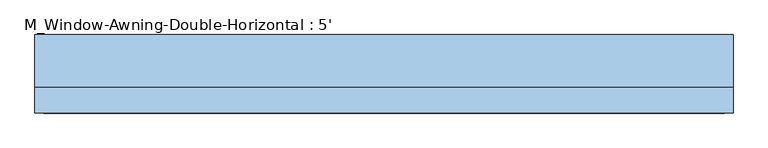
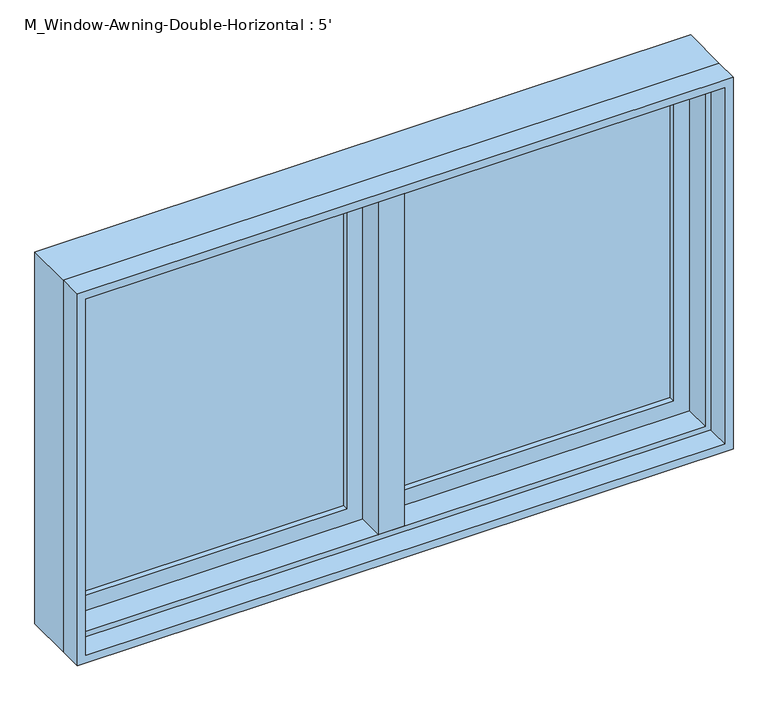
"""IFC4 building model written with IfcOpenShell, lengths in millimetres: window geometry, M_Window-Awning-Double-Horizontal : 5'."""

from ifc_helpers import new_model, si_unit, frame, origin, place, context, project, spatial, polyline, outline, extrude, faceted_brep, source, transform, mapped, element, save


def m_window_awning_double_horizontal_5_337400f2(model_context):
    return source(origin(), model_context, "Body", "SolidModel", [
        faceted_brep([(730.25, 44.45, 1782.65), (730.25, -19.05, 1782.65), (-730.25, -19.05, 1782.65), (-730.25, 44.45, 1782.65), (749.3, 95.25, 1801.7), (749.3, 44.45, 1801.7), (-749.3, 44.45, 1801.7), (-749.3, 95.25, 1801.7), (762.0, -19.05, 1814.4), (762.0, 95.25, 1814.4), (-762.0, 95.25, 1814.4), (-762.0, -19.05, 1814.4), (-730.25, -19.05, 931.75), (-730.25, 44.45, 931.75), (-749.3, 44.45, 912.7), (-749.3, 95.25, 912.7), (-762.0, 95.25, 900.0), (-762.0, -19.05, 900.0), (730.25, -19.05, 931.75), (730.25, 44.45, 931.75), (749.3, 44.45, 912.7), (749.3, 95.25, 912.7), (762.0, 95.25, 900.0), (762.0, -19.05, 900.0)], [[[0, 1, 2, 3]], [[4, 5, 6, 7]], [[8, 9, 10, 11]], [[3, 2, 12, 13]], [[7, 6, 14, 15]], [[11, 10, 16, 17]], [[13, 12, 18, 19]], [[15, 14, 20, 21]], [[17, 16, 22, 23]], [[11, 17, 23, 8], [1, 18, 12, 2]], [[19, 18, 1, 0]], [[5, 20, 14, 6], [3, 13, 19, 0]], [[21, 20, 5, 4]], [[23, 22, 9, 8]], [[9, 22, 16, 10], [7, 15, 21, 4]]]),
        extrude(outline(polyline([(1814.4, -762.0), (900.0, -762.0), (900.0, 762.0), (1814.4, 762.0), (1814.4, -762.0)]), holes=[polyline([(1795.35, 742.95), (919.05, 742.95), (919.05, -742.95), (1795.35, -742.95), (1795.35, 742.95)])]), frame((0.0, -76.2, 0.0), z_axis=(0.0, 1.0, 0.0), x_axis=(0.0, 0.0, 1.0)), (0.0, 0.0, 1.0), 57.15),
        extrude(outline(polyline([(912.7, 749.3), (1801.7, 749.3), (1801.7, 9.525), (912.7, 9.525), (912.7, 749.3)]), holes=[polyline([(969.85, 66.675), (1744.55, 66.675), (1744.55, 692.15), (969.85, 692.15), (969.85, 66.675)])]), frame((0.0, 44.45, 0.0), z_axis=(0.0, 1.0, 0.0), x_axis=(0.0, 0.0, 1.0)), (0.0, 0.0, 1.0), 44.45),
        extrude(outline(polyline([(1801.7, -749.3), (912.7, -749.3), (912.7, -9.525), (1801.7, -9.525), (1801.7, -749.3)]), holes=[polyline([(1744.55, -66.675), (969.85, -66.675), (969.85, -692.15), (1744.55, -692.15), (1744.55, -66.675)])]), frame((0.0, 44.45, 0.0), z_axis=(0.0, 1.0, 0.0), x_axis=(0.0, 0.0, 1.0)), (0.0, 0.0, 1.0), 44.45),
        extrude(outline(polyline([(692.15, 76.2), (692.15, 69.85), (66.675, 69.85), (66.675, 76.2), (692.15, 76.2)])), frame((0.0, 0.0, 969.85), z_axis=(0.0, 0.0, 1.0), x_axis=(1.0, 0.0, 0.0)), (0.0, 0.0, 1.0), 774.7),
        extrude(outline(polyline([(66.675, 57.15), (66.675, 63.5), (692.15, 63.5), (692.15, 57.15), (66.675, 57.15)])), frame((0.0, 0.0, 969.85), z_axis=(0.0, 0.0, 1.0), x_axis=(1.0, 0.0, 0.0)), (0.0, 0.0, 1.0), 774.7),
        extrude(outline(polyline([(-66.675, 76.2), (-66.675, 69.85), (-692.15, 69.85), (-692.15, 76.2), (-66.675, 76.2)])), frame((0.0, 0.0, 969.85), z_axis=(0.0, 0.0, 1.0), x_axis=(1.0, 0.0, 0.0)), (0.0, 0.0, 1.0), 774.7),
        extrude(outline(polyline([(-692.15, 57.15), (-692.15, 63.5), (-66.675, 63.5), (-66.675, 57.15), (-692.15, 57.15)])), frame((0.0, 0.0, 969.85), z_axis=(0.0, 0.0, 1.0), x_axis=(1.0, 0.0, 0.0)), (0.0, 0.0, 1.0), 774.7),
        faceted_brep([(9.525, 95.25, 1801.7), (-9.525, 95.25, 1801.7), (-9.525, 44.45, 1801.7), (9.525, 44.45, 1801.7), (9.525, 95.25, 912.7), (9.525, 44.45, 912.7), (-9.525, 44.45, 912.7), (-9.525, 95.25, 912.7), (-9.525, 44.45, 931.75), (-9.525, 44.45, 1782.65), (-30.1625, 44.45, 931.75), (-30.1625, 44.45, 1782.65), (-30.1625, -19.05, 931.75), (-30.1625, -19.05, 1782.65), (30.1625, -19.05, 931.75), (30.1625, -19.05, 1782.65), (30.1625, 44.45, 931.75), (30.1625, 44.45, 1782.65), (9.525, 44.45, 931.75), (9.525, 44.45, 1782.65)], [[[0, 1, 2, 3]], [[4, 5, 6, 7]], [[1, 0, 4, 7]], [[2, 1, 7, 6, 8, 9]], [[9, 8, 10, 11]], [[11, 10, 12, 13]], [[13, 12, 14, 15]], [[15, 14, 16, 17]], [[17, 16, 18, 19]], [[0, 3, 19, 18, 5, 4]], [[18, 8, 6, 5]], [[9, 19, 3, 2]], [[8, 18, 16, 14, 12, 10]], [[19, 9, 11, 13, 15, 17]]]),
    ])


if __name__ == "__main__":
    model = new_model("IFC4")
    model_context = context("Model", 3, world=origin())
    ifc_project = project(units=[si_unit("LENGTHUNIT", "METRE", prefix="MILLI")], contexts=[model_context])
    site = spatial("IfcSite", under=ifc_project)
    building = spatial("IfcBuilding", under=site)
    placement = place(None, origin())
    m_window_awning_double_horizontal_5_shape = m_window_awning_double_horizontal_5_337400f2(model_context)
    element("IfcWindow", 1, ObjectType="M_Window-Awning-Double-Horizontal : 5'", at=placement, inside=building, context=model_context, shape_type="MappedRepresentation", body=[
        mapped(m_window_awning_double_horizontal_5_shape, transform((0.0, 0.0, 0.0), x_axis=(1.0, 0.0, 0.0), y_axis=(0.0, 1.0, 0.0), z_axis=(0.0, 0.0, 1.0))),
    ])
    save(model, "model.ifc")

# Revit data of these elements
# Type "M_Window-Awning-Double-Horizontal : 5'"
#   Type Mark = "19"
#   Fire Rating = "0.5h"
#   Assembly Code = "B2020100"
#   Analytic Construction = "Double glazing - domestic"
#   Window Inset [instance default] = 0' - 0"
#   Wall Thickness [instance default] = 0' - 5.90551"
#   Interior Wall Closure [instance default] = 0' - 2.15551"
#   Half Width = 2' - 6"
#   Visual Light Transmittance = 0.81
#   Thermal Resistance (R) = 1.8146 (h·ft²·°F)/BTU
#   Solar Heat Gain Coefficient = 0.76
#   Rough Width = 5' - 0.59055"
#   Rough Height = 3' - 0.59055"
#   Height = 3' - 0"
#   Heat Transfer Coefficient (U) = 0.5511 BTU/(h·ft²·°F)
#   Frame Extension [instance default] = 0' - 0 1/4"
#   Exterior Wall Closure [instance default] = 0' - 1 1/4"
#   Extension Jamb [instance default] = 0' - 2.15551"
#   Default Sill Height = 2' - 11.43307"
#   Width = 5' - 0"
#   Muntin Visibility = yes
#   Interior Trim Visibility [instance default] = yes
#   Exterior Trim Visibility [instance default] = yes
#   Extension Jamb Visibility [instance default] = yes
#   Interior Trim Material = Wood - Stained
#   Muntin Pattern = M_Muntin Pattern_2x2 : M_Muntin Pattern_2x2
#   Interior Trim = M_Trim-Window-Interior-Flat : Picture Frame
#   Interior Frame Material = Wood - Stained
#   Glass Panel Material = Glass
#   Exterior Trim Material = Clad - White
#   Exterior Trim = M_Trim-Window-Exterior-Flat : with Sill
#   Exterior Frame Material = Clad - White
#   Wall Closure = (empty or 0)
# Element 1 (IfcWindow, "M_Window-Awning-Double-Horizontal : 5'")
#   Wall Thickness = 0' - 6"
#   Extension Jamb = 0' - 2 1/4"
#   Materials on its faces: "Wood - Stained", "Glass", "Clad - White"
# Materials
#   "Wood - Stained": class "Wood", colour RGB 224 178 126, transparency 0, Cost = 0
#   "Glass": class "Glass", colour RGB 0 128 192, transparency 0.75, Description = "Soda Lime Glass", Cost = 0
#   "Clad - White": class "Wood", colour RGB 242 242 238, transparency 0, Cost = 0
